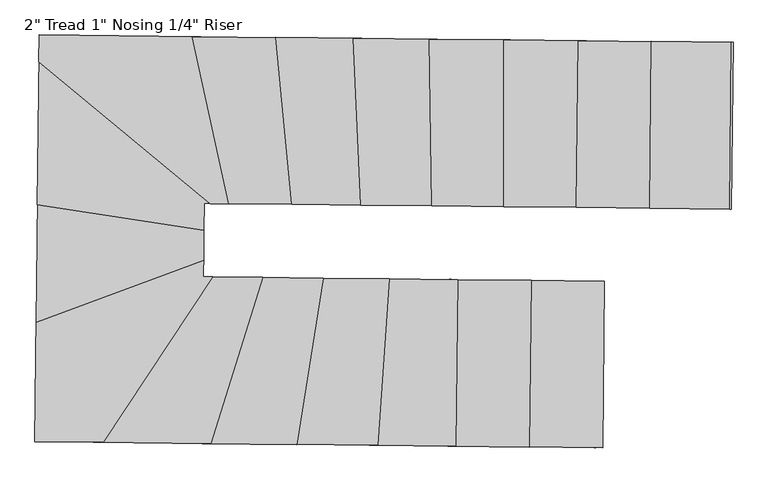
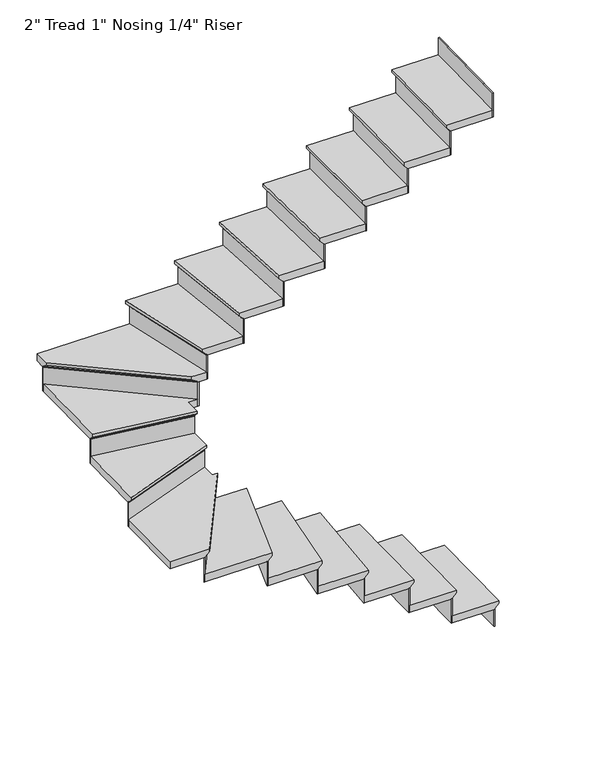
"""IFC4 building model written with IfcOpenShell, lengths in millimetres: stair flight geometry."""

from ifc_helpers import new_model, si_unit, origin, place, context, project, spatial, faceted_brep, source, transform, mapped, element, save


def stair_flight_64b704a5(model_context):
    return source(origin(), model_context, "Body", "Brep", [
        faceted_brep([(-1961.6349602, -4965.4067295, 6551.0833333), (-1961.6349602, -4965.4067295, 6570.1333333), (-1968.4523403, -5600.3701326, 6570.1333333), (-1968.4523403, -5600.3701326, 6551.0833333), (-1987.0334963, -4965.1340343, 6525.6833333), (-1993.8508764, -5600.0974374, 6525.6833333), (-2266.4173937, -4962.134387, 6570.1333333), (-2273.2347738, -5597.0977902, 6570.1333333), (-1993.8508764, -5600.0974374, 6519.3333333), (-2273.2347738, -5597.0977902, 6519.3333333), (-2266.4173937, -4962.134387, 6519.3333333), (-1987.0334963, -4965.1340343, 6519.3333333)], [[[0, 1, 2, 3]], [[4, 0, 3, 5]], [[2, 1, 6, 7]], [[8, 9, 10, 11]], [[2, 7, 9, 8, 5, 3]], [[8, 11, 4, 5]], [[6, 1, 0, 4, 11, 10]], [[7, 6, 10, 9]]]),
        faceted_brep([(-1987.0334963, -4965.1340343, 6519.3333333), (-1987.0334963, -4965.1340343, 6400.8), (-1993.3831304, -4965.0658605, 6400.8), (-1993.3831304, -4965.0658605, 6519.3333333), (-1993.8508764, -5600.0974374, 6519.3333333), (-2000.2005104, -5600.0292636, 6519.3333333), (-2000.2005104, -5600.0292636, 6400.8), (-1993.8508764, -5600.0974374, 6400.8)], [[[0, 1, 2, 3]], [[4, 5, 6, 7]], [[1, 0, 4, 7]], [[2, 1, 7, 6]], [[3, 2, 6, 5]], [[0, 3, 5, 4]]]),
        faceted_brep([(-2266.4173937, -4962.134387, 6688.6666667), (-2266.4173937, -4962.134387, 6519.3333333), (-2272.7670277, -4962.0662132, 6519.3333333), (-2272.7670277, -4962.0662132, 6688.6666667), (-2273.2347738, -5597.0977902, 6688.6666667), (-2279.5844078, -5597.0296164, 6688.6666667), (-2279.5844078, -5597.0296164, 6519.3333333), (-2273.2347738, -5597.0977902, 6519.3333333)], [[[0, 1, 2, 3]], [[4, 5, 6, 7]], [[1, 0, 4, 7]], [[2, 1, 7, 6]], [[3, 2, 6, 5]], [[0, 3, 5, 4]]]),
        faceted_brep([(-2247.8362377, -5597.3704854, 6739.4666667), (-2241.0188576, -4962.4070822, 6739.4666667), (-2545.8012911, -4959.1347398, 6739.4666667), (-2552.6186712, -5594.0981429, 6739.4666667), (-2273.2347738, -5597.0977902, 6688.6666667), (-2552.6186712, -5594.0981429, 6688.6666667), (-2545.8012911, -4959.1347398, 6688.6666667), (-2266.4173937, -4962.134387, 6688.6666667), (-2273.2347738, -5597.0977902, 6695.0166667), (-2247.8362377, -5597.3704854, 6720.4166667), (-2266.4173937, -4962.134387, 6695.0166667), (-2241.0188576, -4962.4070822, 6720.4166667)], [[[0, 1, 2, 3]], [[4, 5, 6, 7]], [[0, 3, 5, 4, 8, 9]], [[4, 7, 10, 8]], [[2, 1, 11, 10, 7, 6]], [[3, 2, 6, 5]], [[11, 1, 0, 9]], [[10, 11, 9, 8]]]),
        faceted_brep([(-2545.8012911, -4959.1347398, 6858.0), (-2545.8012911, -4959.1347398, 6688.6666667), (-2552.1509251, -4959.066566, 6688.6666667), (-2552.1509251, -4959.066566, 6858.0), (-2552.6186712, -5594.0981429, 6858.0), (-2558.9683052, -5594.0299691, 6858.0), (-2558.9683052, -5594.0299691, 6688.6666667), (-2552.6186712, -5594.0981429, 6688.6666667)], [[[0, 1, 2, 3]], [[4, 5, 6, 7]], [[1, 0, 4, 7]], [[2, 1, 7, 6]], [[3, 2, 6, 5]], [[0, 3, 5, 4]]]),
        faceted_brep([(-2527.2201351, -5594.3708381, 6908.8), (-2520.402755, -4959.407435, 6908.8), (-2806.7760852, -4956.3327447, 6908.8), (-2850.4973934, -5590.8999232, 6908.8), (-2552.6186712, -5594.0981429, 6858.0), (-2850.4973934, -5590.8999232, 6858.0), (-2806.7760852, -4956.3327447, 6858.0), (-2545.8012911, -4959.1347398, 6858.0), (-2552.6186712, -5594.0981429, 6864.35), (-2527.2201351, -5594.3708381, 6889.75), (-2545.8012911, -4959.1347398, 6864.35), (-2520.402755, -4959.407435, 6889.75)], [[[0, 1, 2, 3]], [[4, 5, 6, 7]], [[0, 3, 5, 4, 8, 9]], [[4, 7, 10, 8]], [[2, 1, 11, 10, 7, 6]], [[3, 2, 6, 5]], [[11, 1, 0, 9]], [[10, 11, 9, 8]]]),
        faceted_brep([(-2806.7760852, -4956.3327447, 7027.3333333), (-2806.7760852, -4956.3327447, 6858.0), (-2813.1364345, -4956.2644558, 6858.0), (-2813.1364345, -4956.2644558, 7027.3333333), (-2850.4973934, -5590.8999232, 7027.3333333), (-2856.8577426, -5590.8316344, 7027.3333333), (-2856.8577426, -5590.8316344, 6858.0), (-2850.4973934, -5590.8999232, 6858.0)], [[[0, 1, 2, 3]], [[4, 5, 6, 7]], [[1, 0, 4, 7]], [[2, 1, 7, 6]], [[3, 2, 6, 5]], [[0, 3, 5, 4]]]),
        faceted_brep([(-2825.0559965, -5591.1730786, 7078.1333333), (-2781.3346883, -4956.6059001, 7078.1333333), (-3058.0757112, -4953.6346284, 7078.1333333), (-3158.4280189, -5587.5937798, 7078.1333333), (-2850.4973934, -5590.8999232, 7027.3333333), (-3158.4280189, -5587.5937798, 7027.3333333), (-3058.0757112, -4953.6346284, 7027.3333333), (-2806.7760852, -4956.3327447, 7027.3333333), (-2850.4973934, -5590.8999232, 7033.6833333), (-2825.0559965, -5591.1730786, 7059.0833333), (-2806.7760852, -4956.3327447, 7033.6833333), (-2781.3346883, -4956.6059001, 7059.0833333)], [[[0, 1, 2, 3]], [[4, 5, 6, 7]], [[0, 3, 5, 4, 8, 9]], [[4, 7, 10, 8]], [[2, 1, 11, 10, 7, 6]], [[3, 2, 6, 5]], [[11, 1, 0, 9]], [[10, 11, 9, 8]]]),
        faceted_brep([(-3058.0757112, -4953.6346284, 7196.6666667), (-3058.0757112, -4953.6346284, 7027.3333333), (-3064.4938676, -4953.5657189, 7027.3333333), (-3064.4938676, -4953.5657189, 7196.6666667), (-3158.4280189, -5587.5937798, 7196.6666667), (-3164.8461752, -5587.5248703, 7196.6666667), (-3164.8461752, -5587.5248703, 7027.3333333), (-3158.4280189, -5587.5937798, 7027.3333333)], [[[0, 1, 2, 3]], [[4, 5, 6, 7]], [[1, 0, 4, 7]], [[2, 1, 7, 6]], [[3, 2, 6, 5]], [[0, 3, 5, 4]]]),
        faceted_brep([(-3132.7553936, -5587.8694178, 7247.4666667), (-3032.4030859, -4953.9102664, 7247.4666667), (-3289.3424431, -4951.1515984, 7247.4666667), (-3487.6403792, -5584.0591417, 7247.4666667), (-3158.4280189, -5587.5937798, 7196.6666667), (-3487.6403792, -5584.0591417, 7196.6666667), (-3289.3424431, -4951.1515984, 7196.6666667), (-3058.0757112, -4953.6346284, 7196.6666667), (-3158.4280189, -5587.5937798, 7203.0166667), (-3132.7553936, -5587.8694178, 7228.4166667), (-3058.0757112, -4953.6346284, 7203.0166667), (-3032.4030859, -4953.9102664, 7228.4166667)], [[[0, 1, 2, 3]], [[4, 5, 6, 7]], [[0, 3, 5, 4, 8, 9]], [[4, 7, 10, 8]], [[2, 1, 11, 10, 7, 6]], [[3, 2, 6, 5]], [[11, 1, 0, 9]], [[10, 11, 9, 8]]]),
        faceted_brep([(-3289.3424431, -4951.1515984, 7366.0), (-3289.3424431, -4951.1515984, 7196.6666667), (-3295.9745116, -4951.0803922, 7196.6666667), (-3295.9745116, -4951.0803922, 7366.0), (-3487.6403792, -5584.0591417, 7366.0), (-3494.2724477, -5583.9879355, 7366.0), (-3494.2724477, -5583.9879355, 7196.6666667), (-3487.6403792, -5584.0591417, 7196.6666667)], [[[0, 1, 2, 3]], [[4, 5, 6, 7]], [[1, 0, 4, 7]], [[2, 1, 7, 6]], [[3, 2, 6, 5]], [[0, 3, 5, 4]]]),
        faceted_brep([(-3461.1121052, -5584.3439665, 7416.8), (-3262.8141691, -4951.4364232, 7416.8), (-3484.2219113, -4949.0592457, 7416.8), (-3900.4163626, -5579.6273103, 7416.8), (-3487.6403792, -5584.0591417, 7366.0), (-3900.4163626, -5579.6273103, 7366.0), (-3484.2219113, -4949.0592457, 7366.0), (-3289.3424431, -4951.1515984, 7366.0), (-3487.6403792, -5584.0591417, 7372.35), (-3461.1121052, -5584.3439665, 7397.75), (-3289.3424431, -4951.1515984, 7372.35), (-3262.8141691, -4951.4364232, 7397.75)], [[[0, 1, 2, 3]], [[4, 5, 6, 7]], [[0, 3, 5, 4, 8, 9]], [[4, 7, 10, 8]], [[2, 1, 11, 10, 7, 6]], [[3, 2, 6, 5]], [[11, 1, 0, 9]], [[10, 11, 9, 8]]]),
        faceted_brep([(-3484.2219113, -4949.0592457, 7535.3333333), (-3484.2219113, -4949.0592457, 7366.0), (-3491.7768309, -4948.9781311, 7366.0), (-3491.7768309, -4948.9781311, 7535.3333333), (-3900.4163626, -5579.6273103, 7535.3333333), (-3907.9712823, -5579.5461958, 7535.3333333), (-3907.9712823, -5579.5461958, 7366.0), (-3900.4163626, -5579.6273103, 7366.0)], [[[0, 1, 2, 3]], [[4, 5, 6, 7]], [[1, 0, 4, 7]], [[2, 1, 7, 6]], [[3, 2, 6, 5]], [[0, 3, 5, 4]]]),
        faceted_brep([(-4125.8898698, -5095.6676694, 7586.1333333), (-4131.0593878, -5577.1509768, 7586.1333333), (-3870.196684, -5579.9517684, 7586.1333333), (-3454.0022327, -4949.3837038, 7586.1333333), (-3489.2786045, -4949.0049537, 7586.1333333), (-3488.312708, -4859.0423992, 7586.1333333), (-4131.0593878, -5577.1509768, 7535.3333333), (-4125.8898698, -5095.6676694, 7535.3333333), (-3488.312708, -4859.0423992, 7535.3333333), (-3489.2786045, -4949.0049537, 7535.3333333), (-3484.2219113, -4949.0592457, 7535.3333333), (-3900.4163626, -5579.6273103, 7535.3333333), (-3900.4163626, -5579.6273103, 7541.6833333), (-3870.196684, -5579.9517684, 7567.0833333), (-3484.2219113, -4949.0592457, 7541.6833333), (-3454.0022327, -4949.3837038, 7567.0833333)], [[[0, 1, 2, 3, 4, 5]], [[6, 7, 8, 9, 10, 11]], [[1, 0, 7, 6]], [[2, 1, 6, 11, 12, 13]], [[11, 10, 14, 12]], [[4, 3, 15, 14, 10, 9]], [[5, 4, 9, 8]], [[0, 5, 8, 7]], [[15, 3, 2, 13]], [[14, 15, 13, 12]]]),
        faceted_brep([(-3488.312708, -4859.0423992, 7704.6666667), (-3488.312708, -4859.0423992, 7535.3333333), (-3488.2396954, -4852.2420842, 7535.3333333), (-3488.2396954, -4852.2420842, 7704.6666667), (-4125.8898698, -5095.6676694, 7704.6666667), (-4125.8168572, -5088.8673543, 7704.6666667), (-4125.8168572, -5088.8673543, 7535.3333333), (-4125.8898698, -5095.6676694, 7535.3333333)], [[[0, 1, 2, 3]], [[4, 5, 6, 7]], [[1, 0, 4, 7]], [[2, 1, 7, 6]], [[3, 2, 6, 5]], [[0, 3, 5, 4]]]),
        faceted_brep([(-4126.1819202, -5122.8689296, 7755.4666667), (-3488.6047585, -4886.2436594, 7755.4666667), (-3487.1016265, -4746.243576, 7755.4666667), (-4121.0934321, -4648.9326558, 7755.4666667), (-4125.8898698, -5095.6676694, 7704.6666667), (-4121.0934321, -4648.9326558, 7704.6666667), (-3487.1016265, -4746.243576, 7704.6666667), (-3488.312708, -4859.0423992, 7704.6666667), (-4125.8898698, -5095.6676694, 7711.0166667), (-4126.1819202, -5122.8689296, 7736.4166667), (-3488.312708, -4859.0423992, 7711.0166667), (-3488.6047585, -4886.2436594, 7736.4166667)], [[[0, 1, 2, 3]], [[4, 5, 6, 7]], [[0, 3, 5, 4, 8, 9]], [[4, 7, 10, 8]], [[3, 2, 6, 5]], [[11, 1, 0, 9]], [[10, 11, 9, 8]], [[2, 1, 11, 10, 7, 6]]]),
        faceted_brep([(-3487.1016265, -4746.243576, 7874.0), (-3487.1016265, -4746.243576, 7704.6666667), (-3487.0327638, -4739.8297815, 7704.6666667), (-3487.0327638, -4739.8297815, 7874.0), (-4121.0934321, -4648.9326558, 7874.0), (-4121.0245695, -4642.5188612, 7874.0), (-4121.0245695, -4642.5188612, 7704.6666667), (-4121.0934321, -4648.9326558, 7704.6666667)], [[[0, 1, 2, 3]], [[4, 5, 6, 7]], [[1, 0, 4, 7]], [[2, 1, 7, 6]], [[3, 2, 6, 5]], [[0, 3, 5, 4]]]),
        faceted_brep([(-4121.3688828, -4674.587834, 7924.8), (-3487.3770772, -4771.8987542, 7924.8), (-3486.2789573, -4669.6210563, 7924.8), (-3423.6180491, -4670.2938246, 7924.8), (-4115.1699262, -4097.2237198, 7924.8), (-4121.0934321, -4648.9326558, 7874.0), (-4115.1699262, -4097.2237198, 7874.0), (-3423.6180491, -4670.2938246, 7874.0), (-3486.2789573, -4669.6210563, 7874.0), (-3487.1016265, -4746.243576, 7874.0), (-4121.0934321, -4648.9326558, 7880.35), (-4121.3688828, -4674.587834, 7905.75), (-3487.1016265, -4746.243576, 7880.35), (-3487.3770772, -4771.8987542, 7905.75)], [[[0, 1, 2, 3, 4]], [[5, 6, 7, 8, 9]], [[0, 4, 6, 5, 10, 11]], [[5, 9, 12, 10]], [[2, 1, 13, 12, 9, 8]], [[4, 3, 7, 6]], [[13, 1, 0, 11]], [[12, 13, 11, 10]], [[3, 2, 8, 7]]]),
        faceted_brep([(-3423.6180491, -4670.2938246, 8043.3333333), (-3423.6180491, -4670.2938246, 7874.0), (-3413.5354356, -4670.4020781, 7874.0), (-3413.5354356, -4670.4020781, 8043.3333333), (-4115.1699262, -4097.2237198, 8043.3333333), (-4115.0821626, -4089.0495147, 8043.3333333), (-4115.0821626, -4089.0495147, 7874.0), (-4115.1699262, -4097.2237198, 7874.0)], [[[0, 1, 2, 3]], [[4, 5, 6, 7]], [[1, 0, 4, 7]], [[2, 1, 7, 6]], [[3, 2, 6, 5]], [[0, 3, 5, 4]]]),
        faceted_brep([(-3506.4342514, -4034.368057, 8094.1333333), (-4114.4249804, -4027.8402731, 8094.1333333), (-4115.5209805, -4129.9205399, 8094.1333333), (-3463.9485035, -4669.8608106, 8094.1333333), (-3365.8789969, -4670.9137486, 8094.1333333), (-4114.4249804, -4027.8402731, 8043.3333333), (-3506.4342514, -4034.368057, 8043.3333333), (-3365.8789969, -4670.9137486, 8043.3333333), (-3423.6180491, -4670.2938246, 8043.3333333), (-4115.1699262, -4097.2237198, 8043.3333333), (-3423.6180491, -4670.2938246, 8049.6833333), (-4115.1699262, -4097.2237198, 8049.6833333), (-3463.9485035, -4669.8608106, 8075.0833333), (-4115.5209805, -4129.9205399, 8075.0833333)], [[[0, 1, 2, 3, 4]], [[5, 6, 7, 8, 9]], [[1, 0, 6, 5]], [[9, 8, 10, 11]], [[4, 3, 12, 10, 8, 7]], [[0, 4, 7, 6]], [[12, 3, 2, 13]], [[10, 12, 13, 11]], [[2, 1, 5, 9, 11, 13]]]),
        faceted_brep([(-3365.8789969, -4670.9137486, 8212.6666667), (-3365.8789969, -4670.9137486, 8043.3333333), (-3359.3605829, -4670.9837346, 8043.3333333), (-3359.3605829, -4670.9837346, 8212.6666667), (-3506.4342514, -4034.368057, 8212.6666667), (-3499.9158374, -4034.438043, 8212.6666667), (-3499.9158374, -4034.438043, 8043.3333333), (-3506.4342514, -4034.368057, 8043.3333333)], [[[0, 1, 2, 3]], [[4, 5, 6, 7]], [[1, 0, 4, 7]], [[2, 1, 7, 6]], [[3, 2, 6, 5]], [[0, 3, 5, 4]]]),
        faceted_brep([(-3532.5079076, -4034.0881133, 8263.4666667), (-3391.9526531, -4670.6338049, 8263.4666667), (-3127.2086135, -4673.4762691, 8263.4666667), (-3187.4049598, -4037.793363, 8263.4666667), (-3506.4342514, -4034.368057, 8212.6666667), (-3187.4049598, -4037.793363, 8212.6666667), (-3127.2086135, -4673.4762691, 8212.6666667), (-3365.8789969, -4670.9137486, 8212.6666667), (-3506.4342514, -4034.368057, 8219.0166667), (-3532.5079076, -4034.0881133, 8244.4166667), (-3365.8789969, -4670.9137486, 8219.0166667), (-3391.9526531, -4670.6338049, 8244.4166667)], [[[0, 1, 2, 3]], [[4, 5, 6, 7]], [[0, 3, 5, 4, 8, 9]], [[4, 7, 10, 8]], [[2, 1, 11, 10, 7, 6]], [[3, 2, 6, 5]], [[11, 1, 0, 9]], [[10, 11, 9, 8]]]),
        faceted_brep([(-3127.2086135, -4673.4762691, 8382.0), (-3127.2086135, -4673.4762691, 8212.6666667), (-3120.8237144, -4673.5448215, 8212.6666667), (-3120.8237144, -4673.5448215, 8382.0), (-3187.4049598, -4037.793363, 8382.0), (-3181.0200608, -4037.8619154, 8382.0), (-3181.0200608, -4037.8619154, 8212.6666667), (-3187.4049598, -4037.793363, 8212.6666667)], [[[0, 1, 2, 3]], [[4, 5, 6, 7]], [[1, 0, 4, 7]], [[2, 1, 7, 6]], [[3, 2, 6, 5]], [[0, 3, 5, 4]]]),
        faceted_brep([(-3212.9445562, -4037.5191533, 8432.8), (-3152.7482098, -4673.2020594, 8432.8), (-2863.8799111, -4676.3035373, 8432.8), (-2892.1704009, -4040.9631932, 8432.8), (-3187.4049598, -4037.793363, 8382.0), (-2892.1704009, -4040.9631932, 8382.0), (-2863.8799111, -4676.3035373, 8382.0), (-3127.2086135, -4673.4762691, 8382.0), (-3187.4049598, -4037.793363, 8388.35), (-3212.9445562, -4037.5191533, 8413.75), (-3127.2086135, -4673.4762691, 8388.35), (-3152.7482098, -4673.2020594, 8413.75)], [[[0, 1, 2, 3]], [[4, 5, 6, 7]], [[0, 3, 5, 4, 8, 9]], [[4, 7, 10, 8]], [[2, 1, 11, 10, 7, 6]], [[3, 2, 6, 5]], [[11, 1, 0, 9]], [[10, 11, 9, 8]]]),
        faceted_brep([(-2863.8799111, -4676.3035373, 8551.3333333), (-2863.8799111, -4676.3035373, 8382.0), (-2857.5205787, -4676.3718152, 8382.0), (-2857.5205787, -4676.3718152, 8551.3333333), (-2892.1704009, -4040.9631932, 8551.3333333), (-2885.8110685, -4041.0314712, 8551.3333333), (-2885.8110685, -4041.0314712, 8382.0), (-2892.1704009, -4040.9631932, 8382.0)], [[[0, 1, 2, 3]], [[4, 5, 6, 7]], [[1, 0, 4, 7]], [[2, 1, 7, 6]], [[3, 2, 6, 5]], [[0, 3, 5, 4]]]),
        faceted_brep([(-2917.6077305, -4040.6900815, 8602.1333333), (-2889.3172407, -4676.0304256, 8602.1333333), (-2593.0867697, -4679.2109486, 8602.1333333), (-2604.2529652, -4044.0544621, 8602.1333333), (-2892.1704009, -4040.9631932, 8551.3333333), (-2604.2529652, -4044.0544621, 8551.3333333), (-2593.0867697, -4679.2109486, 8551.3333333), (-2863.8799111, -4676.3035373, 8551.3333333), (-2892.1704009, -4040.9631932, 8557.6833333), (-2917.6077305, -4040.6900815, 8583.0833333), (-2863.8799111, -4676.3035373, 8557.6833333), (-2889.3172407, -4676.0304256, 8583.0833333)], [[[0, 1, 2, 3]], [[4, 5, 6, 7]], [[0, 3, 5, 4, 8, 9]], [[4, 7, 10, 8]], [[2, 1, 11, 10, 7, 6]], [[3, 2, 6, 5]], [[11, 1, 0, 9]], [[10, 11, 9, 8]]]),
        faceted_brep([(-2593.0867697, -4679.2109486, 8720.6666667), (-2593.0867697, -4679.2109486, 8551.3333333), (-2586.7345895, -4679.2791497, 8551.3333333), (-2586.7345895, -4679.2791497, 8720.6666667), (-2604.2529652, -4044.0544621, 8720.6666667), (-2597.900785, -4044.1226632, 8720.6666667), (-2597.900785, -4044.1226632, 8551.3333333), (-2604.2529652, -4044.0544621, 8551.3333333)], [[[0, 1, 2, 3]], [[4, 5, 6, 7]], [[1, 0, 4, 7]], [[2, 1, 7, 6]], [[3, 2, 6, 5]], [[0, 3, 5, 4]]]),
        faceted_brep([(-2629.661686, -4043.7816575, 8771.4666667), (-2618.4954904, -4678.9381441, 8771.4666667), (-2319.0528449, -4682.1531551, 8771.4666667), (-2319.536107, -4047.1113675, 8771.4666667), (-2604.2529652, -4044.0544621, 8720.6666667), (-2319.536107, -4047.1113675, 8720.6666667), (-2319.0528449, -4682.1531551, 8720.6666667), (-2593.0867697, -4679.2109486, 8720.6666667), (-2604.2529652, -4044.0544621, 8727.0166667), (-2629.661686, -4043.7816575, 8752.4166667), (-2593.0867697, -4679.2109486, 8727.0166667), (-2618.4954904, -4678.9381441, 8752.4166667)], [[[0, 1, 2, 3]], [[4, 5, 6, 7]], [[0, 3, 5, 4, 8, 9]], [[4, 7, 10, 8]], [[2, 1, 11, 10, 7, 6]], [[3, 2, 6, 5]], [[11, 1, 0, 9]], [[10, 11, 9, 8]]]),
        faceted_brep([(-2319.0528449, -4682.1531551, 8890.0), (-2319.0528449, -4682.1531551, 8720.6666667), (-2312.7027912, -4682.2213334, 8720.6666667), (-2312.7027912, -4682.2213334, 8890.0), (-2319.536107, -4047.1113675, 8890.0), (-2313.1860533, -4047.1795458, 8890.0), (-2313.1860533, -4047.1795458, 8720.6666667), (-2319.536107, -4047.1113675, 8720.6666667)], [[[0, 1, 2, 3]], [[4, 5, 6, 7]], [[1, 0, 4, 7]], [[2, 1, 7, 6]], [[3, 2, 6, 5]], [[0, 3, 5, 4]]]),
        faceted_brep([(-2344.9363219, -4046.8386542, 8940.8), (-2344.4530598, -4681.8804418, 8940.8), (-2043.3209474, -4685.113592, 8940.8), (-2036.5035673, -4050.1501889, 8940.8), (-2319.536107, -4047.1113675, 8890.0), (-2036.5035673, -4050.1501889, 8890.0), (-2043.3209474, -4685.113592, 8890.0), (-2319.0528449, -4682.1531551, 8890.0), (-2319.536107, -4047.1113675, 8896.35), (-2344.9363219, -4046.8386542, 8921.75), (-2319.0528449, -4682.1531551, 8896.35), (-2344.4530598, -4681.8804418, 8921.75)], [[[0, 1, 2, 3]], [[4, 5, 6, 7]], [[0, 3, 5, 4, 8, 9]], [[4, 7, 10, 8]], [[2, 1, 11, 10, 7, 6]], [[3, 2, 6, 5]], [[11, 1, 0, 9]], [[10, 11, 9, 8]]]),
        faceted_brep([(-2043.3209474, -4685.113592, 9059.3333333), (-2043.3209474, -4685.113592, 8890.0), (-2036.9713133, -4685.1817658, 8890.0), (-2036.9713133, -4685.1817658, 9059.3333333), (-2036.5035673, -4050.1501889, 9059.3333333), (-2030.1539332, -4050.2183627, 9059.3333333), (-2030.1539332, -4050.2183627, 8890.0), (-2036.5035673, -4050.1501889, 8890.0)], [[[0, 1, 2, 3]], [[4, 5, 6, 7]], [[1, 0, 4, 7]], [[2, 1, 7, 6]], [[3, 2, 6, 5]], [[0, 3, 5, 4]]]),
        faceted_brep([(-2061.9021034, -4049.8774937, 9110.1333333), (-2068.7194835, -4684.8408968, 9110.1333333), (-1763.93705, -4688.1132393, 9110.1333333), (-1757.1196699, -4053.1498361, 9110.1333333), (-2036.5035673, -4050.1501889, 9059.3333333), (-1757.1196699, -4053.1498361, 9059.3333333), (-1763.93705, -4688.1132393, 9059.3333333), (-2043.3209474, -4685.113592, 9059.3333333), (-2036.5035673, -4050.1501889, 9065.6833333), (-2061.9021034, -4049.8774937, 9091.0833333), (-2043.3209474, -4685.113592, 9065.6833333), (-2068.7194835, -4684.8408968, 9091.0833333)], [[[0, 1, 2, 3]], [[4, 5, 6, 7]], [[0, 3, 5, 4, 8, 9]], [[4, 7, 10, 8]], [[2, 1, 11, 10, 7, 6]], [[3, 2, 6, 5]], [[11, 1, 0, 9]], [[10, 11, 9, 8]]]),
        faceted_brep([(-1763.93705, -4688.1132393, 9228.6666667), (-1763.93705, -4688.1132393, 9059.3333333), (-1757.5874159, -4688.1814131, 9059.3333333), (-1757.5874159, -4688.1814131, 9228.6666667), (-1757.1196699, -4053.1498361, 9228.6666667), (-1750.7700359, -4053.2180099, 9228.6666667), (-1750.7700359, -4053.2180099, 9059.3333333), (-1757.1196699, -4053.1498361, 9059.3333333)], [[[0, 1, 2, 3]], [[4, 5, 6, 7]], [[1, 0, 4, 7]], [[2, 1, 7, 6]], [[3, 2, 6, 5]], [[0, 3, 5, 4]]]),
        faceted_brep([(-1484.5531526, -4691.1128865, 9398.0), (-1484.5531526, -4691.1128865, 9228.6666667), (-1478.2035186, -4691.1810603, 9228.6666667), (-1478.2035186, -4691.1810603, 9398.0), (-1477.7357725, -4056.1494834, 9398.0), (-1471.3861385, -4056.2176572, 9398.0), (-1471.3861385, -4056.2176572, 9228.6666667), (-1477.7357725, -4056.1494834, 9228.6666667)], [[[0, 1, 2, 3]], [[4, 5, 6, 7]], [[1, 0, 4, 7]], [[2, 1, 7, 6]], [[3, 2, 6, 5]], [[0, 3, 5, 4]]]),
        faceted_brep([(-1782.518206, -4052.8771409, 9279.4666667), (-1789.3355861, -4687.8405441, 9279.4666667), (-1484.5531526, -4691.1128865, 9279.4666667), (-1477.7357725, -4056.1494834, 9279.4666667), (-1757.1196699, -4053.1498361, 9228.6666667), (-1477.7357725, -4056.1494834, 9228.6666667), (-1484.5531526, -4691.1128865, 9228.6666667), (-1763.93705, -4688.1132393, 9228.6666667), (-1757.1196699, -4053.1498361, 9235.0166667), (-1782.518206, -4052.8771409, 9260.4166667), (-1763.93705, -4688.1132393, 9235.0166667), (-1789.3355861, -4687.8405441, 9260.4166667)], [[[0, 1, 2, 3]], [[4, 5, 6, 7]], [[0, 3, 5, 4, 8, 9]], [[4, 7, 10, 8]], [[2, 1, 11, 10, 7, 6]], [[3, 2, 6, 5]], [[11, 1, 0, 9]], [[10, 11, 9, 8]]]),
    ])


if __name__ == "__main__":
    model = new_model("IFC4")
    model_context = context("Model", 3, world=origin())
    ifc_project = project(units=[si_unit("LENGTHUNIT", "METRE", prefix="MILLI")], contexts=[model_context])
    site = spatial("IfcSite", under=ifc_project)
    building = spatial("IfcBuilding", under=site)
    placement = place(None, origin())
    stair_flight_shape = stair_flight_64b704a5(model_context)
    element("IfcStairFlight", 1, ObjectType="2\" Tread 1\" Nosing 1/4\" Riser", at=placement, inside=building, context=model_context, shape_type="MappedRepresentation", body=[
        mapped(stair_flight_shape, transform((0.0, 0.0, 0.0), x_axis=(1.0, 0.0, 0.0), y_axis=(0.0, 1.0, 0.0), z_axis=(0.0, 0.0, 1.0))),
    ])
    save(model, "model.ifc")
